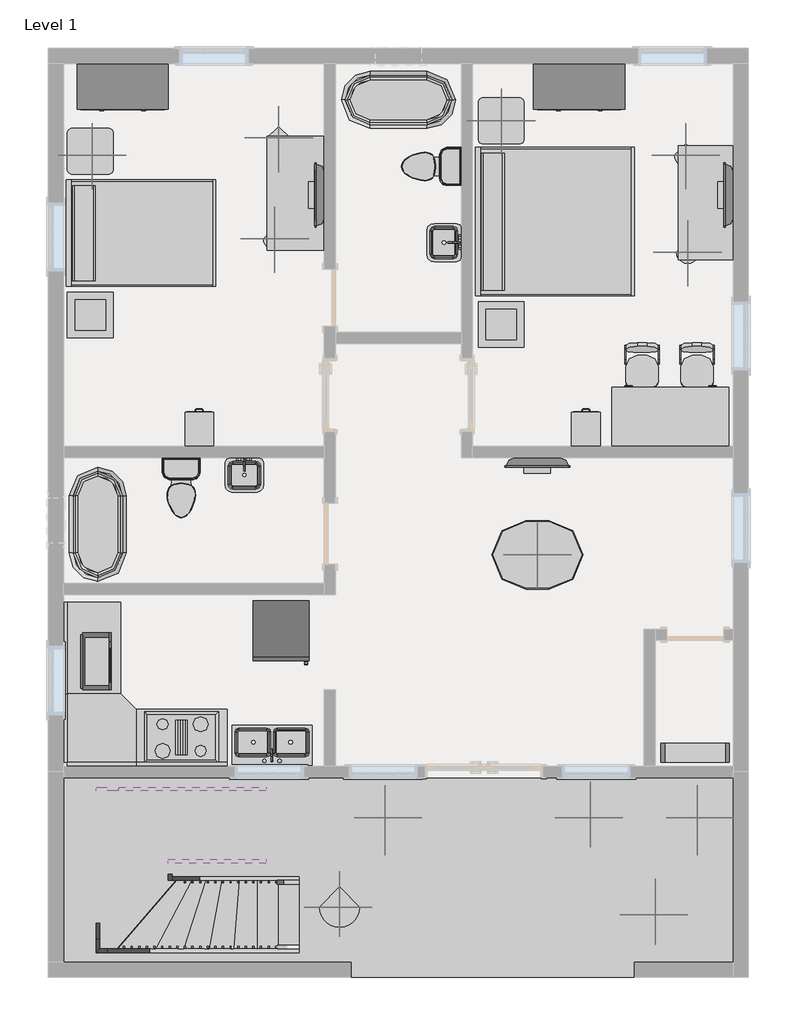
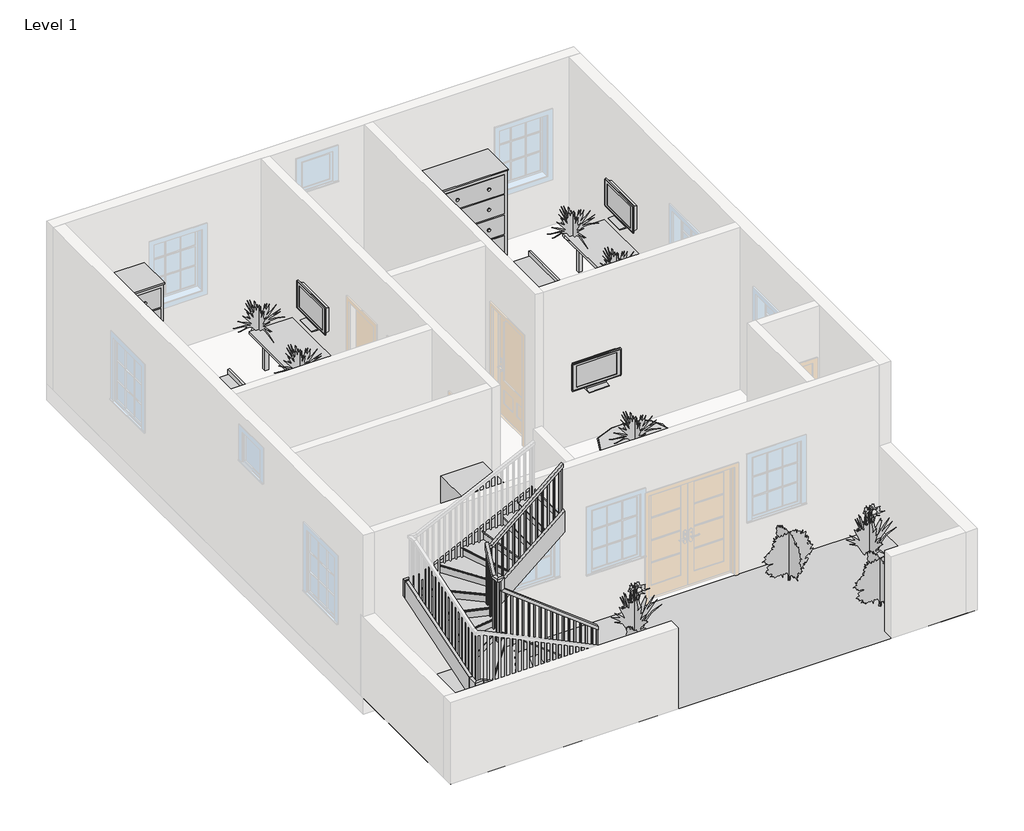
# One storey, part 3 of 3: 21 furniture elements, 12 geographic elements, 9 flow terminals, 9 members, 4 proxies, 1 railing, 1 stair flight.
# Revit data of these elements (continued)
# Materials (continued)
#   "Laminate, Ivory, Matte": class "Plastic", colour RGB 247 247 239, transparency 0, Description = "Plastic Laminate - Ivory, Matte", Cost = 0
#   "Cherry": class "Wood", colour RGB 226 177 128, transparency 0, Description = "Prunus Serotina", Cost = 0
#   "Wood - Teak": class "Wood", colour RGB 145 112 90, transparency 0
#   "Linen, Beige": class "Textile", colour RGB 249 239 230, transparency 0, Description = "Linen, beige", Cost = 0
#   "Steel, Paint Finish, Dark Gray, Matte": class "Metal", colour RGB 0 0 0, transparency 0, Description = "Steel, paint finish, dark gray, matte", Cost = 0
#   "Glass - Clear, Grey": class "Glass", colour RGB 252 255 255, transparency 0.64
#   "Textile - Light Gray": class "Fabric", colour RGB 204 204 204, transparency 0
#   "Plant": class "Generic", colour RGB 0 0 0, transparency 0, Description = "physical material", Cost = 0
#   "Glass": class "Glass", colour RGB 0 128 192, transparency 0.75, Description = "Soda Lime Glass", Cost = 0
#   "TV - Black": colour RGB 49 49 49, transparency 0
#   "TV - Glass": colour RGB 157 157 157, transparency 0.9
#   "TV - Screen": colour RGB 0 0 0, transparency 0
